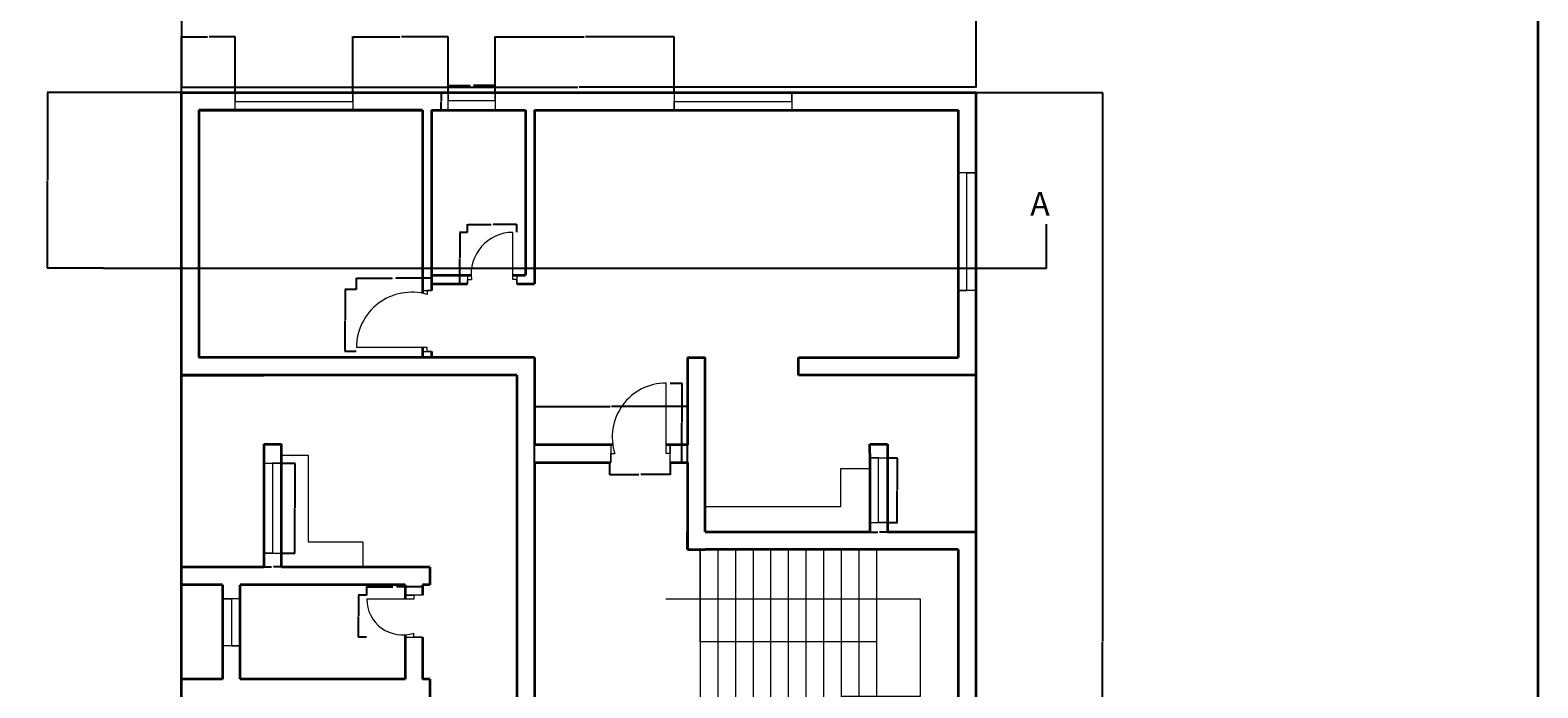
# Model space of a CAD drawing. Units: inches. Extents: x 1955 to 3324, y 980 to 3129.
# Tile 8 of 11: x 2555 to 3324, y 2153 to 2488. Entities that reach past the tile are written whole.
import ezdxf

# ---------------------------------------------------------------- set-up
doc = ezdxf.new("R2010")
doc.units = ezdxf.units.IN
for name, color, linetype, lineweight in [('A-ANNO-DIMS', 2, 'Continuous', 18), ('A-ANNO-SYMB', 2, 'Continuous', 25), ('A-ANNO-TTLB', 7, 'Continuous', 35), ('A-DOOR', 3, 'Continuous', 18), ('A-FLOR-CASE', 8, 'Continuous', 18), ('A-FLOR-STRS', 7, 'Continuous', 18), ('A-GLAZ', 4, 'Continuous', 18), ('A-WALL', 7, 'Continuous', 35), ('A-WALL-PATT', 252, 'Continuous', 13)]:
    doc.layers.add(name, color=color, linetype=linetype, lineweight=lineweight)
doc.styles.get("Standard").update_dxf_attribs({"font": 'arial.ttf'})
doc.dimstyles.get("Standard").update_dxf_attribs({"dimtxt": 0.18, "dimasz": 0.18, "dimexe": 0.18, "dimexo": 0.0625, "dimgap": 0.09, "dimtad": 0, "dimtih": 1, "dimtoh": 1, "dimdec": 4, "dimzin": 0, "dimdsep": 46, "dimtxsty": 'Standard', "dimcen": 0.09, "dimadec": 0, "dimazin": 0, "dimtfac": 1, "dimtdec": 4, "dimtofl": 0, "dimtmove": 0, "dimatfit": 3, "dimfxl": 1, "dimtolj": 1, "dimtzin": 0, "dimarcsym": 0})

# ---------------------------------------------------------------- blocks, each defined once
blk = doc.blocks.new('DOOR-BED-N')
for p, q in [((33.75, 31.05), (38.25, 31.05)), ((38.25, 31.05), (36, 31.05)), ((36, 31.05), (36, 29.05)), ((36, 2), (0, 2)), ((36, 0), (36, 2)), ((33.75, 0), (38.25, 0)), ((38.25, 0), (36, 0))]:
    blk.add_line(p, q)
blk.add_arc((28.16, 2), 28.16, 73.84333, 180)
blk = doc.blocks.new('DOOR-WC-W')
for p, q in [((24, 19.31), (0, 19.31)), ((28.5, 21.31), (19.5, 21.31)), ((19.5, 21.31), (24, 21.31)), ((24, 21.31), (24, 19.31)), ((19.5, 0), (28.5, 0)), ((24, 0), (24, 2)), ((28.5, 0), (24, 0))]:
    blk.add_line(p, q)
blk.add_arc((18.25, 19.31), 18.25, 180, 288.3841)
blk = doc.blocks.new('DOOR-WC-N')
for p, q in [((23.02, 2.25), (23.02, 26.25)), ((0, 4.5), (0, 0)), ((0, 0), (0, 2.25)), ((0, 2.25), (2, 2.25)), ((25.02, 2.25), (23.02, 2.25)), ((25.02, 4.5), (25.02, 0)), ((25.02, 0), (25.02, 2.25))]:
    blk.add_line(p, q)
blk.add_arc((23.02, 5.05), 21.2, 90, 187.58175)
blk = doc.blocks.new('DOOR-UNIT-N')
for p, q in [((28.16, 4.5), (28.16, 40.5)), ((0, 9), (0, 0)), ((30.16, 0), (30.16, 9)), ((30.16, 9), (30.16, 4.5)), ((0, 0), (0, 4.5)), ((0, 4.5), (2, 4.5)), ((30.16, 4.5), (28.16, 4.5))]:
    blk.add_line(p, q)
blk.add_arc((28.16, 12.99), 27.51, 90, 197.98198)
blk = doc.blocks.new('WIN-PLAN-60-A')
for p, q in [((0, 60), (9, 60)), ((9, 60), (4.5, 60)), ((4.5, 60), (4.5, 0)), ((4.5, 0), (0, 0)), ((0, 0), (9, 0))]:
    blk.add_line(p, q)
blk = doc.blocks.new('WIN-PLAN-60-B')
for p, q in [((0, 0), (0, 9)), ((0, 9), (0, 4.5)), ((60, 4.5), (60, 9)), ((60, 9), (60, 0)), ((0, 4.5), (60, 4.5))]:
    blk.add_line(p, q)
blk = doc.blocks.new('WIN-PLAN-60-C')
for p, q in [((0, 9), (0, 0)), ((60, 4.5), (60, 9)), ((60, 9), (60, 9)), ((60, 9), (60, 0)), ((0, 0), (0, 4.5)), ((0, 4.5), (60, 4.5))]:
    blk.add_line(p, q)
blk = doc.blocks.new('WIN-PLAN-24-A')
for p, q in [((0, 9), (0, 0)), ((24, 4.5), (24, 9)), ((24, 9), (24, 0)), ((0, 0), (0, 4.5)), ((0, 4.5), (24, 4.5))]:
    blk.add_line(p, q)
blk = doc.blocks.new('WIN-PLAN-24-B')
for p, q in [((0, 0), (0, 9)), ((0, 9), (0, 4.93)), ((24, 4.93), (24, 9)), ((24, 9), (24, 0)), ((0, 4.93), (24, 4.93))]:
    blk.add_line(p, q)
blk = doc.blocks.new('WIN-PLAN-46')
for p, q in [((0, 45.87), (9, 45.87)), ((9, 45.87), (4.5, 45.87)), ((4.5, 45.87), (4.5, 0)), ((4.5, 0), (0, 0)), ((0, 0), (9, 0))]:
    blk.add_line(p, q)
blk = doc.blocks.new('WIN-PLAN-33')
for p, q in [((4.5, 32.88), (0, 32.88)), ((0, 32.88), (9, 32.88)), ((4.5, 0), (4.5, 32.88)), ((0, 0), (9, 0)), ((9, 0), (4.5, 0))]:
    blk.add_line(p, q)
blk = doc.blocks.new('COUNTER-L-N')
for p, q in [((83.99, 19.45), (69.13, 19.45)), ((69.13, 19.45), (69.13, 0)), ((69.13, 0), (0, 0))]:
    blk.add_line(p, q)
blk = doc.blocks.new('COUNTER-L-W')
for p, q in [((0, 57.19), (13.72, 57.19)), ((13.72, 57.19), (13.72, 12.97)), ((13.72, 12.97), (41.47, 12.97)), ((41.47, 12.97), (41.47, 0))]:
    blk.add_line(p, q)
blk = doc.blocks.new('STAIR-RETURN-FLIGHT')
for p, q in [((17.37, 47), (17.37, 94)), ((17.37, 94), (17.37, 0)), ((26.37, 94), (26.37, 0)), ((35.37, 94), (35.37, 0)), ((44.37, 94), (44.37, 0)), ((53.37, 94), (53.37, 0)), ((62.37, 94), (62.37, 0)), ((71.37, 94), (71.37, 0)), ((80.37, 94), (80.37, 0)), ((89.37, 94), (89.37, 0)), ((98.37, 94), (98.37, 0)), ((107.37, 94), (107.37, 0)), ((0, 68.91), (129.63, 68.91)), ((129.63, 68.91), (129.63, 19.03)), ((107.37, 47), (17.37, 47)), ((129.63, 19.03), (89.37, 19.03))]:
    blk.add_line(p, q)
blk = doc.blocks.new('*D39')
at = {"layer": 'A-ANNO-DIMS', "color": 0, "lineweight": -2, "transparency": 16777216}
for p, q in [((2768.43, 2456.57), (2768.43, 2460.28)), ((2768.61, 2460.1), (2779.59, 2460.1)), ((2792.25, 2460.1), (2781.28, 2460.1)), ((2792.43, 2456.57), (2792.43, 2460.28))]:
    blk.add_line(p, q, dxfattribs=at)
at = {"layer": 'A-ANNO-DIMS', "color": 0, "transparency": 16777216}
for points in [[(2768.61, 2460.13), (2768.61, 2460.07), (2768.43, 2460.1)], [(2792.25, 2460.13), (2792.25, 2460.07), (2792.43, 2460.1)]]:
    blk.add_solid(points, dxfattribs=at)
at = {"layer": 'Defpoints', "color": 0, "transparency": 16777216}
for p in [(2792.43, 2460.1), (2768.43, 2456.5), (2792.43, 2456.5)]:
    blk.add_point(p, dxfattribs=at)
at = {"layer": 'A-ANNO-DIMS', "color": 0, "transparency": 16777216, "insert": (2780.43, 2460.1), "char_height": 0.18, "attachment_point": 5}
blk.add_mtext('\\A1;WIN. 24 TYP.', dxfattribs=at)
blk = doc.blocks.new('*D40')
at = {"layer": 'A-ANNO-DIMS', "color": 0, "lineweight": -2, "transparency": 16777216}
for p, q in [((2768.37, 2456.5), (2764.65, 2456.5)), ((2764.83, 2456.32), (2764.83, 2452.19)), ((2768.37, 2447.5), (2764.65, 2447.5)), ((2764.83, 2447.68), (2764.83, 2451.82))]:
    blk.add_line(p, q, dxfattribs=at)
at = {"layer": 'A-ANNO-DIMS', "color": 0, "transparency": 16777216}
for points in [[(2764.8, 2456.32), (2764.86, 2456.32), (2764.83, 2456.5)], [(2764.8, 2447.68), (2764.86, 2447.68), (2764.83, 2447.5)]]:
    blk.add_solid(points, dxfattribs=at)
at = {"layer": 'Defpoints', "color": 0, "transparency": 16777216}
for p in [(2764.83, 2456.5), (2768.43, 2456.5), (2768.43, 2447.5)]:
    blk.add_point(p, dxfattribs=at)
at = {"layer": 'A-ANNO-DIMS', "color": 0, "transparency": 16777216, "insert": (2764.83, 2452), "char_height": 0.18, "attachment_point": 5}
blk.add_mtext('\\A1;9 TYP.', dxfattribs=at)
blk = doc.blocks.new('*D41')
at = {"layer": 'A-ANNO-DIMS', "color": 0, "lineweight": -2, "transparency": 16777216}
for p, q in [((2683.43, 2267.52), (2690.43, 2267.52)), ((2690.25, 2267.34), (2690.25, 2244.77)), ((2690.25, 2221.83), (2690.25, 2244.4)), ((2683.43, 2221.65), (2690.43, 2221.65))]:
    blk.add_line(p, q, dxfattribs=at)
at = {"layer": 'A-ANNO-DIMS', "color": 0, "transparency": 16777216}
for points in [[(2690.22, 2267.34), (2690.28, 2267.34), (2690.25, 2267.52)], [(2690.22, 2221.83), (2690.28, 2221.83), (2690.25, 2221.65)]]:
    blk.add_solid(points, dxfattribs=at)
at = {"layer": 'Defpoints', "color": 0, "transparency": 16777216}
for p in [(2683.37, 2267.52), (2690.25, 2267.52), (2683.37, 2221.65)]:
    blk.add_point(p, dxfattribs=at)
at = {"layer": 'A-ANNO-DIMS', "color": 0, "transparency": 16777216, "insert": (2690.25, 2244.58), "char_height": 0.18, "attachment_point": 5}
blk.add_mtext('\\A1;WIN. 46 TYP.', dxfattribs=at)
blk = doc.blocks.new('*D42')
at = {"layer": 'A-ANNO-DIMS', "color": 0, "lineweight": -2, "transparency": 16777216}
for p, q in [((2674.37, 2221.59), (2674.37, 2214.59)), ((2683.37, 2221.59), (2683.37, 2214.59)), ((2674.55, 2214.77), (2678.41, 2214.77)), ((2683.19, 2214.77), (2679.33, 2214.77))]:
    blk.add_line(p, q, dxfattribs=at)
at = {"layer": 'A-ANNO-DIMS', "color": 0, "transparency": 16777216}
for points in [[(2674.55, 2214.8), (2674.55, 2214.74), (2674.37, 2214.77)], [(2683.19, 2214.8), (2683.19, 2214.74), (2683.37, 2214.77)]]:
    blk.add_solid(points, dxfattribs=at)
at = {"layer": 'Defpoints', "color": 0, "transparency": 16777216}
for p in [(2674.37, 2221.65), (2683.37, 2221.65), (2683.37, 2214.77)]:
    blk.add_point(p, dxfattribs=at)
at = {"layer": 'A-ANNO-DIMS', "color": 0, "transparency": 16777216, "insert": (2678.87, 2214.77), "char_height": 0.18, "attachment_point": 5}
blk.add_mtext('\\A1;9 TYP.', dxfattribs=at)
blk = doc.blocks.new('*D43')
at = {"layer": 'A-ANNO-DIMS', "color": 0, "lineweight": -2, "transparency": 16777216}
for p, q in [((2992.43, 2270.25), (2997.48, 2270.25)), ((2997.3, 2270.07), (2997.3, 2254)), ((2997.3, 2237.56), (2997.3, 2253.63)), ((2992.43, 2237.38), (2997.48, 2237.38))]:
    blk.add_line(p, q, dxfattribs=at)
at = {"layer": 'A-ANNO-DIMS', "color": 0, "transparency": 16777216}
for points in [[(2997.27, 2270.07), (2997.33, 2270.07), (2997.3, 2270.25)], [(2997.27, 2237.56), (2997.33, 2237.56), (2997.3, 2237.38)]]:
    blk.add_solid(points, dxfattribs=at)
at = {"layer": 'Defpoints', "color": 0, "transparency": 16777216}
for p in [(2992.37, 2270.25), (2997.3, 2270.25), (2992.37, 2237.38)]:
    blk.add_point(p, dxfattribs=at)
at = {"layer": 'A-ANNO-DIMS', "color": 0, "transparency": 16777216, "insert": (2997.3, 2253.82), "char_height": 0.18, "attachment_point": 5}
blk.add_mtext('\\A1;WIN. 33 TYP.', dxfattribs=at)
blk = doc.blocks.new('*D44')
at = {"layer": 'A-ANNO-DIMS', "color": 0, "lineweight": -2, "transparency": 16777216}
for p, q in [((2983.37, 2237.31), (2983.37, 2232.26)), ((2992.37, 2237.31), (2992.37, 2232.26)), ((2983.55, 2232.44), (2987.41, 2232.44)), ((2992.19, 2232.44), (2988.33, 2232.44))]:
    blk.add_line(p, q, dxfattribs=at)
at = {"layer": 'A-ANNO-DIMS', "color": 0, "transparency": 16777216}
for points in [[(2983.55, 2232.47), (2983.55, 2232.41), (2983.37, 2232.44)], [(2992.19, 2232.47), (2992.19, 2232.41), (2992.37, 2232.44)]]:
    blk.add_solid(points, dxfattribs=at)
at = {"layer": 'Defpoints', "color": 0, "transparency": 16777216}
for p in [(2983.37, 2237.38), (2992.37, 2237.38), (2992.37, 2232.44)]:
    blk.add_point(p, dxfattribs=at)
at = {"layer": 'A-ANNO-DIMS', "color": 0, "transparency": 16777216, "insert": (2987.87, 2232.44), "char_height": 0.18, "attachment_point": 5}
blk.add_mtext('\\A1;9 TYP.', dxfattribs=at)
blk = doc.blocks.new('*D59')
at = {"layer": 'A-ANNO-DIMS', "color": 0, "lineweight": -2, "transparency": 16777216}
for p, q in [((2721.62, 2356.13), (2721.62, 2361.99)), ((2721.8, 2361.81), (2739.81, 2361.81)), ((2759.69, 2361.81), (2741.68, 2361.81)), ((2759.87, 2356.13), (2759.87, 2361.99))]:
    blk.add_line(p, q, dxfattribs=at)
at = {"layer": 'A-ANNO-DIMS', "color": 0, "transparency": 16777216}
for points in [[(2721.8, 2361.84), (2721.8, 2361.78), (2721.62, 2361.81)], [(2759.69, 2361.84), (2759.69, 2361.78), (2759.87, 2361.81)]]:
    blk.add_solid(points, dxfattribs=at)
at = {"layer": 'Defpoints', "color": 0, "transparency": 16777216}
for p in [(2759.87, 2361.81), (2721.62, 2356.07), (2759.87, 2356.07)]:
    blk.add_point(p, dxfattribs=at)
at = {"layer": 'A-ANNO-DIMS', "color": 0, "transparency": 16777216, "insert": (2740.74, 2361.81), "char_height": 0.18, "attachment_point": 5}
blk.add_mtext('\\A1;DOOR 38 TYP.', dxfattribs=at)
blk = doc.blocks.new('*D60')
at = {"layer": 'A-ANNO-DIMS', "color": 0, "lineweight": -2, "transparency": 16777216}
for p, q in [((2721.56, 2356.07), (2715.7, 2356.07)), ((2715.88, 2355.89), (2715.88, 2340.49)), ((2715.88, 2324.73), (2715.88, 2340.13)), ((2721.56, 2324.55), (2715.7, 2324.55))]:
    blk.add_line(p, q, dxfattribs=at)
at = {"layer": 'A-ANNO-DIMS', "color": 0, "transparency": 16777216}
for points in [[(2715.85, 2355.89), (2715.91, 2355.89), (2715.88, 2356.07)], [(2715.85, 2324.73), (2715.91, 2324.73), (2715.88, 2324.55)]]:
    blk.add_solid(points, dxfattribs=at)
at = {"layer": 'Defpoints', "color": 0, "transparency": 16777216}
for p in [(2715.88, 2356.07), (2721.62, 2356.07), (2721.62, 2324.55)]:
    blk.add_point(p, dxfattribs=at)
at = {"layer": 'A-ANNO-DIMS', "color": 0, "transparency": 16777216, "insert": (2715.88, 2340.31), "char_height": 0.18, "attachment_point": 5}
blk.add_mtext('\\A1;32 TYP.', dxfattribs=at)
blk = doc.blocks.new('*D61')
at = {"layer": 'A-ANNO-DIMS', "color": 0, "lineweight": -2, "transparency": 16777216}
for p, q in [((2726.9, 2200.29), (2726.9, 2204.69)), ((2727.08, 2204.51), (2740.21, 2204.51)), ((2755.22, 2204.51), (2742.08, 2204.51)), ((2755.4, 2200.29), (2755.4, 2204.69))]:
    blk.add_line(p, q, dxfattribs=at)
at = {"layer": 'A-ANNO-DIMS', "color": 0, "transparency": 16777216}
for points in [[(2727.08, 2204.54), (2727.08, 2204.48), (2726.9, 2204.51)], [(2755.22, 2204.54), (2755.22, 2204.48), (2755.4, 2204.51)]]:
    blk.add_solid(points, dxfattribs=at)
at = {"layer": 'Defpoints', "color": 0, "transparency": 16777216}
for p in [(2726.9, 2200.23), (2755.4, 2204.51), (2755.4, 2200.23)]:
    blk.add_point(p, dxfattribs=at)
at = {"layer": 'A-ANNO-DIMS', "color": 0, "transparency": 16777216, "insert": (2741.15, 2204.51), "char_height": 0.18, "attachment_point": 5}
blk.add_mtext('\\A1;DOOR 29 TYP.', dxfattribs=at)
blk = doc.blocks.new('*D62')
at = {"layer": 'A-ANNO-DIMS', "color": 0, "lineweight": -2, "transparency": 16777216}
for p, q in [((2726.84, 2200.23), (2722.44, 2200.23)), ((2722.62, 2200.05), (2722.62, 2189.75)), ((2722.62, 2179.1), (2722.62, 2189.39)), ((2726.84, 2178.92), (2722.44, 2178.92))]:
    blk.add_line(p, q, dxfattribs=at)
at = {"layer": 'A-ANNO-DIMS', "color": 0, "transparency": 16777216}
for points in [[(2722.59, 2200.05), (2722.65, 2200.05), (2722.62, 2200.23)], [(2722.59, 2179.1), (2722.65, 2179.1), (2722.62, 2178.92)]]:
    blk.add_solid(points, dxfattribs=at)
at = {"layer": 'Defpoints', "color": 0, "transparency": 16777216}
for p in [(2722.62, 2200.23), (2726.9, 2200.23), (2726.9, 2178.92)]:
    blk.add_point(p, dxfattribs=at)
at = {"layer": 'A-ANNO-DIMS', "color": 0, "transparency": 16777216, "insert": (2722.62, 2189.57), "char_height": 0.18, "attachment_point": 5}
blk.add_mtext('\\A1;21 TYP.', dxfattribs=at)
blk = doc.blocks.new('*D69')
at = {"layer": 'A-ANNO-DIMS', "color": 0, "lineweight": -2, "transparency": 16777216}
for p, q in [((2778.26, 2385.25), (2774.2, 2385.25)), ((2774.38, 2385.07), (2774.38, 2372.31)), ((2774.38, 2359.18), (2774.38, 2371.95)), ((2778.26, 2359), (2774.2, 2359))]:
    blk.add_line(p, q, dxfattribs=at)
at = {"layer": 'A-ANNO-DIMS', "color": 0, "transparency": 16777216}
for points in [[(2774.35, 2385.07), (2774.41, 2385.07), (2774.38, 2385.25)], [(2774.35, 2359.18), (2774.41, 2359.18), (2774.38, 2359)]]:
    blk.add_solid(points, dxfattribs=at)
at = {"layer": 'Defpoints', "color": 0, "transparency": 16777216}
for p in [(2774.38, 2385.25), (2778.32, 2385.25), (2778.32, 2359)]:
    blk.add_point(p, dxfattribs=at)
at = {"layer": 'A-ANNO-DIMS', "color": 0, "transparency": 16777216, "insert": (2774.38, 2372.13), "char_height": 0.18, "attachment_point": 5}
blk.add_mtext('\\A1;DOOR 26 TYP.', dxfattribs=at)
blk = doc.blocks.new('*D70')
at = {"layer": 'A-ANNO-DIMS', "color": 0, "lineweight": -2, "transparency": 16777216}
for p, q in [((2778.32, 2385.32), (2778.32, 2389.37)), ((2778.5, 2389.19), (2790.3, 2389.19)), ((2803.16, 2389.19), (2791.36, 2389.19)), ((2803.34, 2385.32), (2803.34, 2389.37))]:
    blk.add_line(p, q, dxfattribs=at)
at = {"layer": 'A-ANNO-DIMS', "color": 0, "transparency": 16777216}
for points in [[(2778.5, 2389.22), (2778.5, 2389.16), (2778.32, 2389.19)], [(2803.16, 2389.22), (2803.16, 2389.16), (2803.34, 2389.19)]]:
    blk.add_solid(points, dxfattribs=at)
at = {"layer": 'Defpoints', "color": 0, "transparency": 16777216}
for p in [(2778.32, 2385.25), (2803.34, 2389.19), (2803.34, 2385.25)]:
    blk.add_point(p, dxfattribs=at)
at = {"layer": 'A-ANNO-DIMS', "color": 0, "transparency": 16777216, "insert": (2790.83, 2389.19), "char_height": 0.18, "attachment_point": 5}
blk.add_mtext('\\A1;25 TYP.', dxfattribs=at)
blk = doc.blocks.new('*D71')
at = {"layer": 'A-ANNO-DIMS', "color": 0, "lineweight": -2, "transparency": 16777216}
for p, q in [((2881.6, 2308.43), (2887.79, 2308.43)), ((2887.61, 2308.25), (2887.61, 2288.36)), ((2887.61, 2268.11), (2887.61, 2288)), ((2881.6, 2267.93), (2887.79, 2267.93))]:
    blk.add_line(p, q, dxfattribs=at)
at = {"layer": 'A-ANNO-DIMS', "color": 0, "transparency": 16777216}
for points in [[(2887.58, 2308.25), (2887.64, 2308.25), (2887.61, 2308.43)], [(2887.58, 2268.11), (2887.64, 2268.11), (2887.61, 2267.93)]]:
    blk.add_solid(points, dxfattribs=at)
at = {"layer": 'Defpoints', "color": 0, "transparency": 16777216}
for p in [(2881.54, 2308.43), (2887.61, 2308.43), (2881.54, 2267.93)]:
    blk.add_point(p, dxfattribs=at)
at = {"layer": 'A-ANNO-DIMS', "color": 0, "transparency": 16777216, "insert": (2887.61, 2288.18), "char_height": 0.18, "attachment_point": 5}
blk.add_mtext('\\A1;ENTRY 41 TYP.', dxfattribs=at)
blk = doc.blocks.new('*D72')
at = {"layer": 'A-ANNO-DIMS', "color": 0, "lineweight": -2, "transparency": 16777216}
for p, q in [((2850.66, 2267.87), (2850.66, 2261.67)), ((2881.54, 2267.87), (2881.54, 2261.67)), ((2850.84, 2261.85), (2865.57, 2261.85)), ((2881.36, 2261.85), (2866.63, 2261.85))]:
    blk.add_line(p, q, dxfattribs=at)
at = {"layer": 'A-ANNO-DIMS', "color": 0, "transparency": 16777216}
for points in [[(2850.84, 2261.88), (2850.84, 2261.82), (2850.66, 2261.85)], [(2881.36, 2261.88), (2881.36, 2261.82), (2881.54, 2261.85)]]:
    blk.add_solid(points, dxfattribs=at)
at = {"layer": 'Defpoints', "color": 0, "transparency": 16777216}
for p in [(2850.66, 2267.93), (2881.54, 2267.93), (2881.54, 2261.85)]:
    blk.add_point(p, dxfattribs=at)
at = {"layer": 'A-ANNO-DIMS', "color": 0, "transparency": 16777216, "insert": (2866.1, 2261.85), "char_height": 0.18, "attachment_point": 5}
blk.add_mtext('\\A1;31 TYP.', dxfattribs=at)
blk = doc.blocks.new('*D94')
at = {"layer": 'A-ANNO-DIMS', "color": 0, "lineweight": -2, "transparency": 16777216}
for p, q in [((3037.43, 2456.5), (3102.13, 2456.5)), ((3101.95, 2456.32), (3101.95, 2176.69)), ((3101.95, 1896.68), (3101.95, 2176.32)), ((3037.43, 1896.5), (3102.13, 1896.5))]:
    blk.add_line(p, q, dxfattribs=at)
at = {"layer": 'A-ANNO-DIMS', "color": 0, "transparency": 16777216}
for points in [[(3101.92, 2456.32), (3101.98, 2456.32), (3101.95, 2456.5)], [(3101.92, 1896.68), (3101.98, 1896.68), (3101.95, 1896.5)]]:
    blk.add_solid(points, dxfattribs=at)
at = {"layer": 'Defpoints', "color": 0, "transparency": 16777216}
for p in [(3037.37, 2456.5), (3101.95, 2456.5), (3037.37, 1896.5)]:
    blk.add_point(p, dxfattribs=at)
at = {"layer": 'A-ANNO-DIMS', "color": 0, "transparency": 16777216, "insert": (3101.95, 2176.5), "char_height": 0.18, "attachment_point": 5}
blk.add_mtext('\\A1;560', dxfattribs=at)
blk = doc.blocks.new('*D95')
at = {"layer": 'A-ANNO-DIMS', "color": 0, "lineweight": -2, "transparency": 16777216}
for p, q in [((2632.37, 2456.57), (2632.37, 2485.13)), ((2632.55, 2484.95), (2645.71, 2484.95)), ((2659.66, 2484.95), (2646.5, 2484.95)), ((2659.84, 2456.57), (2659.84, 2485.13))]:
    blk.add_line(p, q, dxfattribs=at)
at = {"layer": 'A-ANNO-DIMS', "color": 0, "transparency": 16777216}
for points in [[(2632.55, 2484.98), (2632.55, 2484.92), (2632.37, 2484.95)], [(2659.66, 2484.98), (2659.66, 2484.92), (2659.84, 2484.95)]]:
    blk.add_solid(points, dxfattribs=at)
at = {"layer": 'Defpoints', "color": 0, "transparency": 16777216}
for p in [(2659.84, 2484.95), (2632.37, 2456.5), (2659.84, 2456.5)]:
    blk.add_point(p, dxfattribs=at)
at = {"layer": 'A-ANNO-DIMS', "color": 0, "transparency": 16777216, "insert": (2646.1, 2484.95), "char_height": 0.18, "attachment_point": 5}
blk.add_mtext('\\A1;27.47', dxfattribs=at)
blk = doc.blocks.new('*D96')
at = {"layer": 'A-ANNO-DIMS', "color": 0, "lineweight": -2, "transparency": 16777216}
for p, q in [((2719.84, 2456.57), (2719.84, 2485.13)), ((2720.02, 2484.95), (2743.74, 2484.95)), ((2768.25, 2484.95), (2744.53, 2484.95)), ((2768.43, 2456.57), (2768.43, 2485.13))]:
    blk.add_line(p, q, dxfattribs=at)
at = {"layer": 'A-ANNO-DIMS', "color": 0, "transparency": 16777216}
for points in [[(2720.02, 2484.98), (2720.02, 2484.92), (2719.84, 2484.95)], [(2768.25, 2484.98), (2768.25, 2484.92), (2768.43, 2484.95)]]:
    blk.add_solid(points, dxfattribs=at)
at = {"layer": 'Defpoints', "color": 0, "transparency": 16777216}
for p in [(2768.43, 2484.95), (2719.84, 2456.5), (2768.43, 2456.5)]:
    blk.add_point(p, dxfattribs=at)
at = {"layer": 'A-ANNO-DIMS', "color": 0, "transparency": 16777216, "insert": (2744.14, 2484.95), "char_height": 0.18, "attachment_point": 5}
blk.add_mtext('\\A1;48.59', dxfattribs=at)
blk = doc.blocks.new('*D97')
at = {"layer": 'A-ANNO-DIMS', "color": 0, "lineweight": -2, "transparency": 16777216}
for p, q in [((2792.43, 2456.57), (2792.43, 2485.13)), ((2792.61, 2484.95), (2837.71, 2484.95)), ((2883.46, 2484.95), (2838.36, 2484.95)), ((2883.64, 2456.57), (2883.64, 2485.13))]:
    blk.add_line(p, q, dxfattribs=at)
at = {"layer": 'A-ANNO-DIMS', "color": 0, "transparency": 16777216}
for points in [[(2792.61, 2484.98), (2792.61, 2484.92), (2792.43, 2484.95)], [(2883.46, 2484.98), (2883.46, 2484.92), (2883.64, 2484.95)]]:
    blk.add_solid(points, dxfattribs=at)
at = {"layer": 'Defpoints', "color": 0, "transparency": 16777216}
for p in [(2883.64, 2484.95), (2792.43, 2456.5), (2883.64, 2456.5)]:
    blk.add_point(p, dxfattribs=at)
at = {"layer": 'A-ANNO-DIMS', "color": 0, "transparency": 16777216, "insert": (2838.04, 2484.95), "char_height": 0.18, "attachment_point": 5}
blk.add_mtext('\\A1;91.2', dxfattribs=at)
blk = doc.blocks.new('*D100')
at = {"layer": 'A-ANNO-DIMS', "color": 0, "lineweight": -2, "transparency": 16777216}
for p, q in [((2632.31, 2456.5), (2564.03, 2456.5)), ((2564.21, 2456.32), (2564.21, 2411.91)), ((2564.21, 2367.13), (2564.21, 2411.54)), ((2592.6, 2366.95), (2564.03, 2366.95))]:
    blk.add_line(p, q, dxfattribs=at)
at = {"layer": 'A-ANNO-DIMS', "color": 0, "transparency": 16777216}
for points in [[(2564.18, 2456.32), (2564.24, 2456.32), (2564.21, 2456.5)], [(2564.18, 2367.13), (2564.24, 2367.13), (2564.21, 2366.95)]]:
    blk.add_solid(points, dxfattribs=at)
at = {"layer": 'Defpoints', "color": 0, "transparency": 16777216}
for p in [(2564.21, 2456.5), (2632.37, 2456.5), (2592.66, 2366.95)]:
    blk.add_point(p, dxfattribs=at)
at = {"layer": 'A-ANNO-DIMS', "color": 0, "transparency": 16777216, "insert": (2564.21, 2411.72), "char_height": 0.18, "attachment_point": 5}
blk.add_mtext('\\A1;89.56', dxfattribs=at)
blk = doc.blocks.new('*D102')
at = {"layer": 'A-ANNO-DIMS', "color": 0, "lineweight": -2, "transparency": 16777216}
for p, q in [((2812.37, 2267.99), (2812.37, 2296.56)), ((2812.55, 2296.38), (2851, 2296.38)), ((2890.2, 2296.38), (2851.75, 2296.38)), ((2890.38, 2267.99), (2890.38, 2296.56))]:
    blk.add_line(p, q, dxfattribs=at)
at = {"layer": 'A-ANNO-DIMS', "color": 0, "transparency": 16777216}
for points in [[(2812.55, 2296.41), (2812.55, 2296.35), (2812.37, 2296.38)], [(2890.2, 2296.41), (2890.2, 2296.35), (2890.38, 2296.38)]]:
    blk.add_solid(points, dxfattribs=at)
at = {"layer": 'Defpoints', "color": 0, "transparency": 16777216}
for p in [(2890.38, 2296.38), (2812.37, 2267.93), (2890.38, 2267.93)]:
    blk.add_point(p, dxfattribs=at)
at = {"layer": 'A-ANNO-DIMS', "color": 0, "transparency": 16777216, "insert": (2851.38, 2296.38), "char_height": 0.18, "attachment_point": 5}
blk.add_mtext('\\A1;78.01', dxfattribs=at)
blk = doc.blocks.new('*D132')
at = {"layer": 'A-ANNO-DIMS', "color": 0, "lineweight": -2, "transparency": 16777216}
for p, q in [((2632.37, 2538.35), (2632.37, 2459.05)), ((3037.37, 2538.35), (3037.37, 2459.05)), ((2632.55, 2459.23), (2834.58, 2459.23)), ((3037.19, 2459.23), (2835.16, 2459.23))]:
    blk.add_line(p, q, dxfattribs=at)
at = {"layer": 'A-ANNO-DIMS', "color": 0, "transparency": 16777216}
for points in [[(2632.55, 2459.26), (2632.55, 2459.2), (2632.37, 2459.23)], [(3037.19, 2459.26), (3037.19, 2459.2), (3037.37, 2459.23)]]:
    blk.add_solid(points, dxfattribs=at)
at = {"layer": 'Defpoints', "color": 0, "transparency": 16777216}
for p in [(2632.37, 2538.41), (3037.37, 2538.41), (3037.37, 2459.23)]:
    blk.add_point(p, dxfattribs=at)
at = {"layer": 'A-ANNO-DIMS', "color": 0, "transparency": 16777216, "insert": (2834.87, 2459.23), "char_height": 0.18, "attachment_point": 5}
blk.add_mtext('\\A1;405', dxfattribs=at)

msp = doc.modelspace()

# ---------------------------------------------------------------- hatches: boundary and pattern name
at = {"layer": 'A-WALL-PATT'}
h = msp.add_hatch(dxfattribs=at)
h.set_pattern_fill('ANSI32', color=256)
h.paths.add_polyline_path([(2361.4775, 2456.5037), (2270.2755, 2456.5037), (2270.2755, 2447.5037), (2285.7102, 2447.5037), (2285.7102, 2363.5037), (2281.1795, 2363.5037), (2281.1795, 2359.0037), (2290.2102, 2359.0037), (2290.2102, 2447.5037), (2361.4775, 2447.5037), (2361.4775, 2452.0037)])
h.paths.add_polyline_path([(2246.2755, 2456.5037), (2197.6809, 2456.5037), (2197.6809, 2447.5037), (2233.2102, 2447.5037), (2233.2102, 2355.6044), (2237.7102, 2355.6044), (2237.7102, 2447.5037), (2246.2755, 2447.5037)], flags=17)
h.paths.add_polyline_path([(2137.6809, 2456.5037), (2110.2102, 2456.5037), (2110.2102, 2312.5037), (2152.2102, 2312.5037), (2281.2102, 2312.5037), (2281.2102, 2107.6185), (2290.2102, 2107.6185), (2290.2102, 2267.9289), (2329.216, 2267.9289), (2329.216, 2272.4289), (2329.216, 2276.9289), (2290.2102, 2276.9289), (2290.2102, 2321.5037), (2281.2102, 2321.5037), (2119.2102, 2321.5037), (2119.2102, 2447.5037), (2137.6809, 2447.5037)])
h.paths.add_polyline_path([(2515.2102, 2456.5037), (2421.4775, 2456.5037), (2421.4775, 2447.5037), (2506.2102, 2447.5037), (2506.2102, 2415.6626), (2515.2102, 2415.6626)])
h.paths.add_polyline_path([(2515.2102, 2355.6626), (2506.2102, 2355.6626), (2506.2102, 2321.5037), (2424.9282, 2321.5037), (2424.9282, 2312.5037), (2461.2102, 2312.5037), (2470.2102, 2312.5037), (2515.2102, 2312.5037)])
h.paths.add_polyline_path([(2515.2102, 2232.5037), (2470.2102, 2232.5037), (2470.2102, 2237.3759), (2465.7102, 2237.3759), (2461.2102, 2237.3759), (2461.2102, 2232.5037), (2377.2219, 2232.5037), (2377.2219, 2321.5037), (2368.2219, 2321.5037), (2368.2219, 2276.9289), (2359.3802, 2276.9289), (2359.3802, 2272.4289), (2359.3802, 2267.9289), (2368.2219, 2267.9289), (2368.2219, 2223.5037), (2377.2219, 2223.5037), (2461.2102, 2223.5037), (2506.2102, 2223.5037), (2506.2102, 2129.5037), (2461.2102, 2129.5037), (2387.2102, 2129.5037), (2368.2219, 2129.5037), (2368.2219, 2056.4936), (2361.0095, 2056.4936), (2361.0095, 2051.9936), (2361.0095, 2047.4936), (2368.2219, 2047.4936), (2368.2219, 2031.5037), (2377.2219, 2031.5037), (2377.2219, 2120.5037), (2461.2102, 2120.5037), (2461.2102, 2112.7921), (2470.2102, 2112.7921), (2470.2102, 2120.5037), (2515.2102, 2120.5037), (2515.2102, 2129.5037)])
h.paths.add_polyline_path([(2470.2102, 2277.1758), (2461.2102, 2277.1758), (2461.2102, 2272.5037), (2461.2102, 2270.2549), (2470.2102, 2270.2549), (2470.2102, 2272.5037)], flags=17)
h.paths.add_polyline_path([(2515.2102, 2040.5037), (2470.2102, 2040.5037), (2417.8264, 2040.5037), (2417.8264, 2031.5037), (2506.2102, 2031.5037), (2506.2102, 2005.3639), (2515.2102, 2005.3639)])
h.paths.add_polyline_path([(2506.2102, 1905.5037), (2402.6963, 1905.5037), (2402.6963, 1896.5037), (2506.2102, 1896.5037)])
h.paths.add_polyline_path([(2515.2102, 1945.3639), (2506.2102, 1945.3639), (2506.2102, 1905.5037), (2506.2102, 1896.5037), (2515.2102, 1896.5037)])
h.paths.add_polyline_path([(2342.6963, 1901.0037), (2342.6963, 1905.5037), (2273.4892, 1905.5037), (2273.4892, 1896.5037), (2342.6963, 1896.5037)])
h.paths.add_polyline_path([(2290.2102, 1994.0037), (2283.612, 1994.0037), (2283.612, 1991.7537), (2283.612, 1989.5037), (2285.7102, 1989.5037), (2285.7102, 1905.5037), (2290.2102, 1905.5037)])
h.paths.add_polyline_path([(2249.4892, 1905.5037), (2237.7102, 1905.5037), (2206.3617, 1905.5037), (2206.3617, 1896.5037), (2249.4892, 1896.5037), (2249.4892, 1901.0037)])
h.paths.add_polyline_path([(2237.7102, 1989.5037), (2261.7102, 1989.5037), (2261.7102, 1994.0037), (2237.7102, 1994.0037), (2237.7102, 1999.266), (2235.4602, 1999.266), (2233.2102, 1999.266), (2233.2102, 1994.0037), (2233.2102, 1905.5037), (2237.7102, 1905.5037)])
h.paths.add_polyline_path([(2119.2102, 1947.5144), (2110.2102, 1947.5144), (2110.2102, 1896.5037), (2119.2102, 1896.5037), (2146.3617, 1896.5037), (2146.3617, 1901.0037), (2146.3617, 1905.5037), (2119.2102, 1905.5037)])
h.paths.add_polyline_path([(2119.2102, 2068.6379), (2110.2102, 2068.6379), (2110.2102, 2007.5144), (2119.2102, 2007.5144), (2119.2102, 2031.5037), (2233.2102, 2031.5037), (2233.2102, 2027.9287), (2235.4602, 2027.9287), (2237.7102, 2027.9287), (2237.7102, 2031.5037), (2281.2102, 2031.5037), (2290.2102, 2031.5037), (2290.2102, 2047.4936), (2326.409, 2047.4936), (2326.409, 2056.4936), (2290.2102, 2056.4936), (2290.2102, 2071.2722), (2285.7102, 2071.2722), (2281.2102, 2071.2722), (2281.2102, 2040.5037), (2227.2102, 2040.5037), (2227.2102, 2111.2571), (2222.7102, 2111.2571), (2218.2102, 2111.2571), (2218.2102, 2040.5037), (2119.2102, 2040.5037)])
h.paths.add_polyline_path([(2236.9166, 2214.5037), (2161.2102, 2214.5037), (2161.2102, 2221.6488), (2152.2102, 2221.6488), (2152.2102, 2214.5037), (2110.2102, 2214.5037), (2110.2102, 2205.5037), (2131.2394, 2205.5037), (2131.2394, 2198.3478), (2140.2394, 2198.3478), (2140.2394, 2205.5037), (2224.2394, 2205.5037), (2224.2394, 2200.2317), (2228.7394, 2200.2317), (2233.2394, 2200.2317), (2233.2394, 2205.5037), (2236.9166, 2205.5037)], flags=17)
h.paths.add_polyline_path([(2236.9166, 2157.5037), (2233.2394, 2157.5037), (2233.2394, 2178.9172), (2228.7394, 2178.9172), (2224.2394, 2178.9172), (2224.2394, 2157.5037), (2140.2394, 2157.5037), (2140.2394, 2174.3478), (2131.2394, 2174.3478), (2131.2394, 2157.5037), (2110.2102, 2157.5037), (2110.2102, 2128.6379), (2119.2102, 2128.6379), (2119.2102, 2148.5037), (2218.2102, 2148.5037), (2218.2102, 2141.7262), (2222.7102, 2141.7262), (2227.2102, 2141.7262), (2227.2102, 2148.5037), (2236.9166, 2148.5037)], flags=0)
h.paths.add_polyline_path([(3084.7449, 2537.3808), (3212.7954, 2537.3808), (3212.7954, 2555.9271), (3084.7449, 2555.9271)], flags=9)
h.paths.add_polyline_path([(3068.7485, 2853.43), (3169.977, 2853.43), (3169.977, 2871.9764), (3068.7485, 2871.9764)], flags=9)
h.paths.add_polyline_path([(3074.1798, 2918.0252), (3126.4732, 2918.0252), (3126.4732, 2936.5716), (3074.1798, 2936.5716)], flags=9)
h.paths.add_polyline_path([(3073.0928, 2947.3127), (3199.0499, 2947.3127), (3199.0499, 2965.8591), (3073.0928, 2965.8591)], flags=9)
h.paths.add_polyline_path([(2733.8393, 2484.8678), (2879.7915, 2484.8678), (2879.7915, 2521.9606), (2733.8393, 2521.9606)], flags=9)
h.paths.add_polyline_path([(2204.9881, 2482.4168), (2355.1272, 2482.4168), (2355.1272, 2519.5095), (2204.9881, 2519.5095)], flags=9)
h.paths.add_polyline_path([(3062.1429, 2387.2466), (3079.3735, 2387.2466), (3079.3735, 2411.9751), (3062.1429, 2411.9751)], flags=9)
h.paths.add_polyline_path([(2190.1574, 2158.8439), (2219.315, 2158.8439), (2219.315, 2177.5013), (2190.1574, 2177.5013)], flags=25)
h.paths.add_polyline_path([(2213.6766, 1840.7276), (2405.0382, 1840.7276), (2405.0382, 1865.4561), (2213.6766, 1865.4561)], flags=9)
h.paths.add_polyline_path([(2180.5398, 2233.911), (2213.9471, 2233.911), (2213.9471, 2252.5683), (2180.5398, 2252.5683)], flags=25)
h.paths.add_polyline_path([(2134.4484, 2238.3973), (2134.4484, 2274.2807), (2115.791, 2274.2807), (2115.791, 2238.3973)], flags=25)
h.paths.add_polyline_path([(2135.1593, 2122.9991), (2173.7507, 2122.9991), (2173.7507, 2141.6565), (2135.1593, 2141.6565)], flags=25)
h.paths.add_polyline_path([(2129.8822, 2002.1912), (2168.4736, 2002.1912), (2168.4736, 2020.8486), (2129.8822, 2020.8486)], flags=9)
h.paths.add_polyline_path([(2239.6647, 1953.4107), (2268.8973, 1953.4107), (2268.8973, 1972.068), (2239.6647, 1972.068)], flags=9)
h.paths.add_polyline_path([(2352.8562, 1951.2904), (2402.1775, 1951.2904), (2402.1775, 1969.9477), (2352.8562, 1969.9477)], flags=9)
h.paths.add_polyline_path([(2500.1358, 2055.32), (2500.1358, 2091.2034), (2481.4784, 2091.2034), (2481.4784, 2055.32)], flags=25)
h.paths.add_polyline_path([(2391.2702, 2058.6821), (2424.4285, 2058.6821), (2424.4285, 2077.3394), (2391.2702, 2077.3394)], flags=25)
h.paths.add_polyline_path([(2507.7996, 2257.2758), (2507.7996, 2293.1592), (2489.1422, 2293.1592), (2489.1422, 2257.2758)], flags=25)
h.paths.add_polyline_path([(2386.8349, 2273.8734), (2419.9931, 2273.8734), (2419.9931, 2292.5307), (2386.8349, 2292.5307)], flags=25)
h.paths.add_polyline_path([(2335.374, 2373.3267), (2384.6953, 2373.3267), (2384.6953, 2391.984), (2335.374, 2391.984)], flags=9)
h.paths.add_polyline_path([(2243.8205, 2380.6539), (2273.0531, 2380.6539), (2273.0531, 2399.3113), (2243.8205, 2399.3113)], flags=25)
h.paths.add_polyline_path([(2126.2627, 2321.6894), (2164.8541, 2321.6894), (2164.8541, 2340.3467), (2126.2627, 2340.3467)], flags=25)

# ---------------------------------------------------------------- linework, layer by layer
at = {"layer": 'A-ANNO-SYMB'}
for p, q in [((3073.4979, 2366.946), (3073.4979, 2389.4136)), ((3073.4979, 2389.4136), (3073.4979, 2389.4136)), ((2592.6595, 2366.946), (3073.4979, 2366.946)), ((3073.4979, 2366.946), (3073.4979, 2366.946))]:
    msp.add_line(p, q, dxfattribs=at)
at = {"layer": 'A-ANNO-TTLB'}
msp.add_lwpolyline([(1954.5391, 3128.9103), (3323.9705, 3128.9103), (3323.9705, 1703.6826), (1954.5391, 1703.6826)], close=True, dxfattribs=at)
at = {"layer": 'A-WALL'}
for p, q in [((2632.3694, 2456.5037), (3037.3694, 2456.5037)), ((2632.3694, 1896.5037), (2632.3694, 2456.5037)), ((3037.3694, 2456.5037), (3037.3694, 1896.5037)), ((2641.3694, 2447.5037), (2755.3694, 2447.5037)), ((2755.3694, 2447.5037), (2641.3694, 2447.5037)), ((2641.3694, 2447.5037), (2641.3694, 2321.5037)), ((2755.3694, 2447.5037), (2755.3694, 2354.157)), ((2759.8694, 2447.5037), (2807.8694, 2447.5037)), ((2759.8694, 2447.5037), (2759.8694, 2355.6044)), ((2807.8694, 2447.5037), (2807.8694, 2363.5037)), ((2812.3694, 2447.5037), (3028.3694, 2447.5037)), ((2812.3694, 2447.5037), (2812.3694, 2359.0037)), ((3028.3694, 2447.5037), (3028.3694, 2321.5037)), ((2759.8694, 2363.5037), (2780.1432, 2363.5037)), ((2801.3387, 2363.5037), (2807.8694, 2363.5037)), ((2759.8694, 2359.0037), (2778.3215, 2359.0037)), ((2803.3387, 2359.0037), (2812.3694, 2359.0037)), ((2812.3694, 2321.5037), (2641.3694, 2321.5037)), ((2755.3694, 2326.5535), (2755.3694, 2321.5037)), ((2759.8694, 2324.5535), (2759.8694, 2321.5037)), ((2812.3694, 2321.5037), (2803.3694, 2321.5037)), ((2812.3694, 2321.5037), (2812.3694, 2276.9289)), ((2890.381, 2321.5037), (2899.381, 2321.5037)), ((2890.381, 2321.5037), (2890.381, 2276.9289)), ((2899.381, 2232.5037), (2899.381, 2321.5037)), ((2947.0873, 2321.5037), (3028.3694, 2321.5037)), ((2947.0873, 2312.5037), (2947.0873, 2321.5037)), ((2803.3694, 2312.5037), (2632.3694, 2312.5037)), ((2632.3694, 2312.5037), (2674.3694, 2312.5037)), ((2803.3694, 2312.5037), (2803.3694, 2105.7875)), ((2983.3694, 2312.5037), (2947.0873, 2312.5037)), ((2992.3694, 2312.5037), (2983.3694, 2312.5037)), ((3037.3694, 2312.5037), (2992.3694, 2312.5037)), ((2674.3694, 2277.1758), (2674.3694, 2214.5037)), ((2674.3694, 2277.1758), (2683.3694, 2277.1758)), ((2683.3694, 2214.5037), (2683.3694, 2277.1758)), ((2852.3227, 2276.9289), (2812.3694, 2276.9289)), ((2890.381, 2276.9289), (2879.5394, 2276.9289)), ((2983.3694, 2272.5037), (2983.3694, 2277.1758)), ((2983.3694, 2277.1758), (2992.3694, 2277.1758)), ((2992.3694, 2277.1758), (2992.3694, 2272.5037)), ((2812.3694, 2267.9289), (2812.3694, 2107.6185)), ((2812.3694, 2267.9289), (2851.3752, 2267.9289)), ((2881.5394, 2267.9289), (2890.381, 2267.9289)), ((2890.381, 2267.9289), (2890.381, 2223.5037)), ((2983.3694, 2272.5037), (2983.3694, 2232.5037)), ((2992.3694, 2272.5037), (2992.3694, 2232.5037)), ((2890.381, 2223.5037), (2890.381, 2232.5037)), ((2899.381, 2232.5037), (2983.3694, 2232.5037)), ((2992.3694, 2232.5037), (3037.3694, 2232.5037)), ((2890.381, 2228.0037), (2890.381, 2223.5037)), ((2890.381, 2223.5037), (2899.381, 2223.5037)), ((2983.3694, 2223.5037), (2899.381, 2223.5037)), ((3028.3694, 2223.5037), (2983.3694, 2223.5037)), ((3028.3694, 2223.5037), (3028.3694, 2129.5037)), ((2674.3694, 2214.5037), (2632.3694, 2214.5037)), ((2759.0757, 2214.5037), (2683.3694, 2214.5037)), ((2759.0757, 2214.5037), (2759.0757, 2205.5037)), ((2653.3985, 2205.5037), (2632.3694, 2205.5037)), ((2653.3985, 2205.5037), (2653.3985, 2157.5037)), ((2746.3985, 2205.5037), (2662.3985, 2205.5037)), ((2662.3985, 2157.5037), (2662.3985, 2205.5037)), ((2746.3985, 2205.5037), (2746.3985, 2198.2317)), ((2759.0757, 2205.5037), (2755.3985, 2205.5037)), ((2755.3985, 2205.5037), (2755.3985, 2200.2317)), ((2746.3985, 2180.0292), (2746.3985, 2157.5037)), ((2755.3985, 2178.9172), (2755.3985, 2157.5037)), ((2653.3985, 2157.5037), (2632.3694, 2157.5037)), ((2746.3985, 2157.5037), (2662.3985, 2157.5037)), ((2746.3985, 2157.5037), (2662.3985, 2157.5037)), ((2759.0757, 2157.5037), (2755.3985, 2157.5037)), ((2759.0757, 2157.5037), (2759.0757, 2148.5037))]:
    msp.add_line(p, q, dxfattribs=at)

# ---------------------------------------------------------------- block references
at = {"layer": 'A-DOOR'}
for name, p in [('DOOR-WC-N', (2778.3211, 2359.004)), ('DOOR-BED-N', (2721.6191, 2324.554)), ('DOOR-UNIT-N', (2851.3751, 2267.929)), ('DOOR-WC-W', (2726.8981, 2178.917))]:
    msp.add_blockref(name, p, dxfattribs=at)
at = {"layer": 'A-FLOR-CASE'}
for name, p in [('COUNTER-L-W', (2683.3691, 2214.504)), ('COUNTER-L-N', (2899.3811, 2245.258))]:
    msp.add_blockref(name, p, dxfattribs=at)
at = {"layer": 'A-FLOR-STRS'}
msp.add_blockref('STAIR-RETURN-FLIGHT', (2879.4531, 2129.504), dxfattribs=at)
at = {"layer": 'A-GLAZ'}
for name, p in [('WIN-PLAN-60-B', (2659.8401, 2447.504)), ('WIN-PLAN-24-B', (2768.4341, 2447.504)), ('WIN-PLAN-60-C', (2883.6371, 2447.504)), ('WIN-PLAN-33', (2983.3691, 2237.376)), ('WIN-PLAN-46', (2674.3691, 2221.649))]:
    msp.add_blockref(name, p, dxfattribs=at)
for name, p, rotation in [('WIN-PLAN-60-A', (3037.3696, 2415.6621), 180), ('WIN-PLAN-24-A', (2653.3988, 2198.3479), 270.0000000000017)]:
    msp.add_blockref(name, p, dxfattribs=dict(at, rotation=rotation))

# ---------------------------------------------------------------- texts
at = {"layer": 'A-ANNO-SYMB', "insert": (3065.1675, 2405.7991), "char_height": 12, "attachment_point": 1}
msp.add_mtext_dynamic_manual_height_columns('A', width=45.337371, gutter_width=12.5, heights=[0], dxfattribs=at)

# ---------------------------------------------------------------- dimensions: what is measured, and where the dimension line sits
at = {"layer": 'A-ANNO-DIMS'}
for base, p1, p2, override, picture, middle in [((3037.3694, 2459.2253), (2632.3694, 2538.4103), (3037.3694, 2538.4103), {"dimdec": 0, "dimlfac": 1, "dimrnd": 0, "dimzin": 0, "dimdsep": 46, "dimlunit": 2}, '*D132', (2834.8694, 2459.2253)), ((2659.84, 2484.9537), (2632.3694, 2456.5037), (2659.84, 2456.5037), {"dimdec": 2, "dimlfac": 1, "dimrnd": 0, "dimzin": 0, "dimdsep": 46, "dimlunit": 2}, '*D95', (2646.1047, 2484.9537)), ((2768.4346, 2484.9537), (2719.84, 2456.5037), (2768.4346, 2456.5037), {"dimdec": 2, "dimlfac": 1, "dimrnd": 0, "dimzin": 0, "dimdsep": 46, "dimlunit": 2}, '*D96', (2744.1373, 2484.9537)), ((2883.6367, 2484.9537), (2792.4346, 2456.5037), (2883.6367, 2456.5037), {"dimdec": 1, "dimlfac": 1, "dimrnd": 0, "dimzin": 0, "dimdsep": 46, "dimlunit": 2}, '*D97', (2838.0356, 2484.9537)), ((2890.381, 2296.3789), (2812.3694, 2267.9289), (2890.381, 2267.9289), {"dimdec": 2, "dimlfac": 1, "dimrnd": 0, "dimzin": 0, "dimdsep": 46, "dimlunit": 2}, '*D102', (2851.3752, 2296.3789))]:
    dim = msp.add_linear_dim(base=base, p1=p1, p2=p2, dimstyle='Standard', override=override, dxfattribs=at)
    dim.commit()
    dim.dimension.update_dxf_attribs({"geometry": picture, "text_midpoint": middle})
for base, p1, p2, text, picture, middle in [((2792.4346, 2460.1037), (2768.4346, 2456.5037), (2792.4346, 2456.5037), 'WIN. <> TYP.', '*D39', (2780.4346, 2460.1037)), ((2803.3387, 2389.1912), (2778.3215, 2385.2537), (2803.3387, 2385.2537), '<> TYP.', '*D70', (2790.8301, 2389.1912)), ((2759.8694, 2361.8061), (2721.6194, 2356.0686), (2759.8694, 2356.0686), 'DOOR <> TYP.', '*D59', (2740.7444, 2361.8061)), ((2881.5394, 2261.8539), (2850.6573, 2267.9289), (2881.5394, 2267.9289), '<> TYP.', '*D72', (2866.0983, 2261.8539)), ((2992.3694, 2232.4441), (2983.3694, 2237.3759), (2992.3694, 2237.3759), '<> TYP.', '*D44', (2987.8694, 2232.4441)), ((2683.3694, 2214.768), (2674.3694, 2221.6488), (2683.3694, 2221.6488), '<> TYP.', '*D42', (2678.8694, 2214.768)), ((2755.3984981169, 2204.5066565334), (2726.8984981169, 2200.2316565334), (2755.3984981169, 2200.2316565334), 'DOOR <> TYP.', '*D61', (2741.1484981169, 2204.5066565334))]:
    dim = msp.add_linear_dim(base=base, p1=p1, p2=p2, text=text, dimstyle='Standard', override={"dimdec": 0, "dimlfac": 1, "dimrnd": 0, "dimzin": 0, "dimdsep": 46, "dimlunit": 2}, dxfattribs=at)
    dim.commit()
    dim.dimension.update_dxf_attribs({"geometry": picture, "text_midpoint": middle})
for base, p1, p2, override, picture, middle in [((2564.2095, 2456.5037), (2592.6595, 2366.946), (2632.3694, 2456.5037), {"dimdec": 2, "dimlfac": 1, "dimrnd": 0, "dimzin": 0, "dimdsep": 46, "dimlunit": 2}, '*D100', (2564.2095, 2411.7248)), ((3101.9479, 2456.5037), (3037.3694, 1896.5037), (3037.3694, 2456.5037), {"dimdec": 0, "dimlfac": 1, "dimrnd": 0, "dimzin": 0, "dimdsep": 46, "dimlunit": 2}, '*D94', (3101.9479, 2176.5037))]:
    dim = msp.add_linear_dim(base=base, p1=p1, p2=p2, angle=90, dimstyle='Standard', override=override, dxfattribs=at)
    dim.commit()
    dim.dimension.update_dxf_attribs({"geometry": picture, "text_midpoint": middle})
for base, p1, p2, text, picture, middle in [((2764.8346, 2456.5037), (2768.4346, 2447.5037), (2768.4346, 2456.5037), '<> TYP.', '*D40', (2764.8346, 2452.0037)), ((2774.384, 2385.2537), (2778.3215, 2359.0037), (2778.3215, 2385.2537), 'DOOR <> TYP.', '*D69', (2774.384, 2372.1287)), ((2715.8819, 2356.0686), (2721.6194, 2324.5535), (2721.6194, 2356.0686), '<> TYP.', '*D60', (2715.8819, 2340.3111)), ((2887.614356255, 2308.4288543301), (2881.539356255, 2267.9288543301), (2881.539356255, 2308.4288543301), 'ENTRY <> TYP.', '*D71', (2887.614356255, 2288.1788543301)), ((2997.3012, 2270.2549), (2992.3694, 2237.3759), (2992.3694, 2270.2549), 'WIN. <> TYP.', '*D43', (2997.3012, 2253.8154)), ((2690.2502, 2267.5208), (2683.3694, 2221.6488), (2683.3694, 2267.5208), 'WIN. <> TYP.', '*D41', (2690.2502, 2244.5848)), ((2722.6235, 2200.2317), (2726.8985, 2178.9172), (2726.8985, 2200.2317), '<> TYP.', '*D62', (2722.6235, 2189.5745))]:
    dim = msp.add_linear_dim(base=base, p1=p1, p2=p2, angle=90, text=text, dimstyle='Standard', override={"dimdec": 0, "dimlfac": 1, "dimrnd": 0, "dimzin": 0, "dimdsep": 46, "dimlunit": 2}, dxfattribs=at)
    dim.commit()
    dim.dimension.update_dxf_attribs({"geometry": picture, "text_midpoint": middle})

doc.saveas('drawing.dxf')
